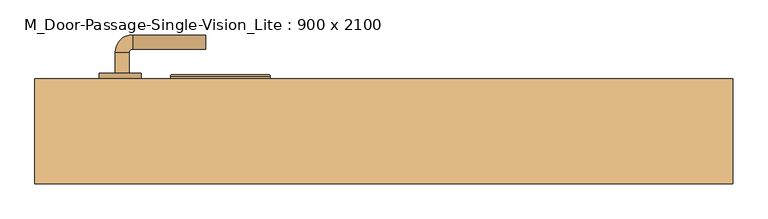
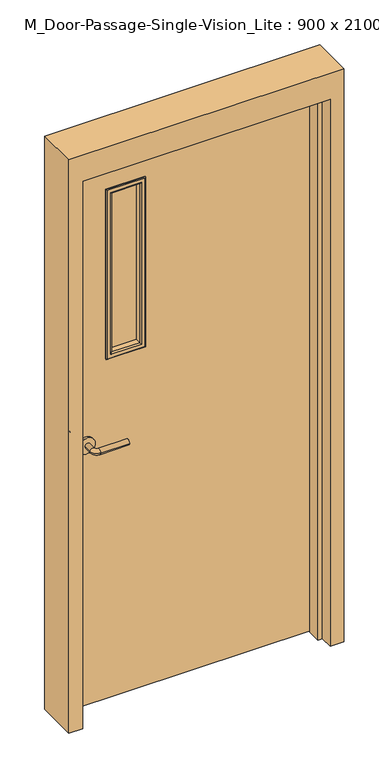
"""IFC4 building model written with IfcOpenShell, lengths in millimetres: door geometry, M_Door-Passage-Single-Vision_Lite : 900 x 2100."""

from ifc_helpers import new_model, si_unit, point, frame, frame_2d, origin, place, context, project, spatial, polyline, circle_curve, ellipse_curve, trimmed, segment, composite_curve, outline, extrude, faceted_brep, source, transform, mapped, element, save
from ifc_brep_helpers import plane_surface, cylinder_surface, revolved_surface, advanced_brep


def m_door_passage_single_vision_lite_900_x_2100_15962226(model_context):
    return source(origin(), model_context, "Body", "SolidModel", [
        advanced_brep(
        [(-384.990625, 40.85, 1000.0), (-364.990625, 40.85, 1000.0), (-364.990625, 10.85, 1000.0), (-384.990625, 10.85, 1000.0), (-359.990625, 5.85, 1000.0), (-359.990625, -14.15, 1000.0), (-254.990625, -14.15, 1000.0), (-254.990625, 5.85, 1000.0)],
        [
            (0, 1, circle_curve(frame((-374.990625, 40.85, 1000.0), z_axis=(0.0, 1.0, 0.0), x_axis=(1.0, 0.0, 0.0)), 10.0)),
            (1, 0, circle_curve(frame((-374.990625, 40.85, 1000.0), z_axis=(0.0, 1.0, 0.0), x_axis=(1.0, 0.0, 0.0)), 10.0)),
            (1, 2),
            (2, 3, circle_curve(frame((-374.990625, 10.85, 1000.0), z_axis=(0.0, 1.0, 0.0), x_axis=(1.0, 0.0, 0.0)), 10.0)),
            (3, 0),
            (3, 2, circle_curve(frame((-374.990625, 10.85, 1000.0), z_axis=(0.0, 1.0, 0.0), x_axis=(1.0, 0.0, 0.0)), 10.0)),
            (4, 5, circle_curve(frame((-359.990625, -4.15, 1000.0), z_axis=(-1.0, 0.0, 0.0), x_axis=(0.0, 1.0, 0.0)), 10.0)),
            (5, 3, circle_curve(frame((-359.990625, 10.85, 1000.0), z_axis=(0.0, 0.0, -1.0), x_axis=(-1.0, 0.0, 0.0)), 25.0)),
            (2, 4, circle_curve(frame((-359.990625, 10.85, 1000.0), z_axis=(0.0, 0.0, 1.0), x_axis=(-1.0, 0.0, 0.0)), 5.0)),
            (5, 4, circle_curve(frame((-359.990625, -4.15, 1000.0), z_axis=(-1.0, 0.0, 0.0), x_axis=(0.0, 1.0, 0.0)), 10.0)),
            (6, 7, circle_curve(frame((-254.990625, -4.15, 1000.0), z_axis=(1.0, 0.0, 0.0), x_axis=(0.0, 1.0, 0.0)), 10.0)),
            (7, 6, circle_curve(frame((-254.990625, -4.15, 1000.0), z_axis=(1.0, 0.0, 0.0), x_axis=(0.0, 1.0, 0.0)), 10.0)),
            (4, 7),
            (6, 5),
        ],
        [
            plane_surface(frame((-374.990625, 40.85, 1000.0), z_axis=(0.0, 1.0, 0.0), x_axis=(0.0, 0.0, 1.0))),
            cylinder_surface(frame((-374.990625, 40.85, 1000.0), z_axis=(0.0, 1.0, 0.0), x_axis=(1.0, 0.0, 0.0)), 10.0),
            revolved_surface(trimmed(ellipse_curve(frame((-374.990625, 10.85, 1000.0), z_axis=(0.0, -1.0, 0.0), x_axis=(1.0, 0.0, 0.0)), 10.0, 10.0), [point((-384.990625, 10.85, 1000.0))], [point((-364.990625, 10.85, 1000.0))], True, "CARTESIAN"), (-359.990625, 10.85, 1000.0), (0.0, 0.0, -1.0)),
            revolved_surface(trimmed(ellipse_curve(frame((-374.990625, 10.85, 1000.0), z_axis=(0.0, -1.0, 0.0), x_axis=(1.0, 0.0, 0.0)), 10.0, 10.0), [point((-364.990625, 10.85, 1000.0))], [point((-384.990625, 10.85, 1000.0))], True, "CARTESIAN"), (-359.990625, 10.85, 1000.0), (0.0, 0.0, -1.0)),
            plane_surface(frame((-254.990625, -4.15, 1000.0), z_axis=(1.0, 0.0, 0.0), x_axis=(0.0, 0.0, 1.0))),
            cylinder_surface(frame((-359.990625, -4.15, 1000.0), z_axis=(-1.0, 0.0, 0.0), x_axis=(0.0, 1.0, 0.0)), 10.0),
        ],
        [
            (0, [[1, 2]]),
            (1, [[3, 4, 5, -2]]),
            (1, [[-5, 6, -3, -1]]),
            (2, [[7, 8, -4, 9]]),
            (3, [[10, -9, -6, -8]]),
            (4, [[11, 12]]),
            (5, [[13, -11, 14, -7]]),
            (5, [[-14, -12, -13, -10]]),
        ],
    ),
        extrude(outline(composite_curve([segment(trimmed(circle_curve(frame_2d((1000.0, -377.490625)), 30.0), [point((1000.0, -407.490625))], [point((1000.0, -347.490625))], False, "CARTESIAN"), True, "CONTINUOUS"), segment(trimmed(circle_curve(frame_2d((1000.0, -377.490625)), 30.0), [point((1000.0, -347.490625))], [point((1000.0, -407.490625))], False, "CARTESIAN"), True, "CONTINUOUS")], self_intersect=False)), frame((0.0, 40.85, 0.0), z_axis=(0.0, 1.0, 0.0), x_axis=(0.0, 0.0, 1.0)), (0.0, 0.0, 1.0), 8.0),
        advanced_brep(
        [(-384.990625, 101.85, 1000.0), (-364.990625, 101.85, 1000.0), (-384.990625, 131.85, 1000.0), (-364.990625, 131.85, 1000.0), (-359.990625, 136.85, 1000.0), (-359.990625, 156.85, 1000.0), (-254.990625, 156.85, 1000.0), (-254.990625, 136.85, 1000.0)],
        [
            (0, 1, circle_curve(frame((-374.990625, 101.85, 1000.0), z_axis=(0.0, -1.0, 0.0), x_axis=(1.0, 0.0, 0.0)), 10.0)),
            (1, 0, circle_curve(frame((-374.990625, 101.85, 1000.0), z_axis=(0.0, -1.0, 0.0), x_axis=(1.0, 0.0, 0.0)), 10.0)),
            (0, 2),
            (2, 3, circle_curve(frame((-374.990625, 131.85, 1000.0), z_axis=(0.0, -1.0, 0.0), x_axis=(1.0, 0.0, 0.0)), 10.0)),
            (3, 1),
            (3, 2, circle_curve(frame((-374.990625, 131.85, 1000.0), z_axis=(0.0, -1.0, 0.0), x_axis=(1.0, 0.0, 0.0)), 10.0)),
            (4, 3, circle_curve(frame((-359.990625, 131.85, 1000.0), z_axis=(0.0, 0.0, 1.0), x_axis=(-1.0, 0.0, 0.0)), 5.0)),
            (2, 5, circle_curve(frame((-359.990625, 131.85, 1000.0), z_axis=(0.0, 0.0, -1.0), x_axis=(-1.0, 0.0, 0.0)), 25.0)),
            (5, 4, circle_curve(frame((-359.990625, 146.85, 1000.0), z_axis=(-1.0, 0.0, 0.0), x_axis=(0.0, -1.0, 0.0)), 10.0)),
            (4, 5, circle_curve(frame((-359.990625, 146.85, 1000.0), z_axis=(-1.0, 0.0, 0.0), x_axis=(0.0, -1.0, 0.0)), 10.0)),
            (6, 7, circle_curve(frame((-254.990625, 146.85, 1000.0), z_axis=(1.0, 0.0, 0.0), x_axis=(0.0, -1.0, 0.0)), 10.0)),
            (7, 6, circle_curve(frame((-254.990625, 146.85, 1000.0), z_axis=(1.0, 0.0, 0.0), x_axis=(0.0, -1.0, 0.0)), 10.0)),
            (5, 6),
            (7, 4),
        ],
        [
            plane_surface(frame((-374.990625, 101.85, 1000.0), z_axis=(0.0, -1.0, 0.0), x_axis=(0.0, 0.0, 1.0))),
            cylinder_surface(frame((-374.990625, 101.85, 1000.0), z_axis=(0.0, -1.0, 0.0), x_axis=(1.0, 0.0, 0.0)), 10.0),
            revolved_surface(trimmed(ellipse_curve(frame((-374.990625, 131.85, 1000.0), z_axis=(0.0, -1.0, 0.0), x_axis=(1.0, 0.0, 0.0)), 10.0, 10.0), [point((-384.990625, 131.85, 1000.0))], [point((-364.990625, 131.85, 1000.0))], True, "CARTESIAN"), (-359.990625, 131.85, 1000.0), (0.0, 0.0, -1.0)),
            revolved_surface(trimmed(ellipse_curve(frame((-374.990625, 131.85, 1000.0), z_axis=(0.0, -1.0, 0.0), x_axis=(1.0, 0.0, 0.0)), 10.0, 10.0), [point((-364.990625, 131.85, 1000.0))], [point((-384.990625, 131.85, 1000.0))], True, "CARTESIAN"), (-359.990625, 131.85, 1000.0), (0.0, 0.0, -1.0)),
            plane_surface(frame((-254.990625, 146.85, 1000.0), z_axis=(1.0, 0.0, 0.0), x_axis=(0.0, 0.0, 1.0))),
            cylinder_surface(frame((-359.990625, 146.85, 1000.0), z_axis=(-1.0, 0.0, 0.0), x_axis=(0.0, -1.0, 0.0)), 10.0),
        ],
        [
            (0, [[1, 2]]),
            (1, [[-1, 3, 4, 5]]),
            (1, [[-2, -5, 6, -3]]),
            (2, [[7, -4, 8, 9]]),
            (3, [[-8, -6, -7, 10]]),
            (4, [[11, 12]]),
            (5, [[-9, 13, -12, 14]]),
            (5, [[-10, -14, -11, -13]]),
        ],
    ),
        extrude(outline(composite_curve([segment(trimmed(circle_curve(frame_2d((1000.0, -377.490625)), 30.0), [point((1000.0, -407.490625))], [point((1000.0, -347.490625))], False, "CARTESIAN"), True, "CONTINUOUS"), segment(trimmed(circle_curve(frame_2d((1000.0, -377.490625)), 30.0), [point((1000.0, -347.490625))], [point((1000.0, -407.490625))], False, "CARTESIAN"), True, "CONTINUOUS")], self_intersect=False)), frame((0.0, 93.85, 0.0), z_axis=(0.0, 1.0, 0.0), x_axis=(0.0, 0.0, 1.0)), (0.0, 0.0, 1.0), 8.0),
        extrude(outline(polyline([(2100.0, -450.0), (0.0, -450.0), (0.0, 450.0), (2100.0, 450.0), (2100.0, -450.0)]), holes=[polyline([(1947.6, -297.6), (1947.6, -170.6), (1312.6, -170.6), (1312.6, -297.6), (1947.6, -297.6)])]), frame((0.0, 48.85, 0.0), z_axis=(0.0, 1.0, 0.0), x_axis=(0.0, 0.0, 1.0)), (0.0, 0.0, 1.0), 45.0),
        faceted_brep([(450.0, 44.0875, 0.0), (450.0, 93.85, 0.0), (500.0, 93.85, 0.0), (500.0, -56.15, 0.0), (450.0, -56.15, 0.0), (450.0, -6.9375, 0.0), (434.125, -6.9375, 0.0), (434.125, 44.0875, 0.0), (450.0, 44.0875, 2100.0), (450.0, 93.85, 2100.0), (-450.0, 93.85, 2100.0), (-450.0, 93.85, 0.0), (-500.0, 93.85, 0.0), (-500.0, 93.85, 2200.0), (500.0, 93.85, 2200.0), (500.0, -56.15, 2200.0), (-500.0, -56.15, 2200.0), (-500.0, -56.15, 0.0), (-450.0, -56.15, 0.0), (-450.0, -56.15, 2100.0), (450.0, -56.15, 2100.0), (450.0, -6.9375, 2100.0), (-450.0, -6.9375, 2100.0), (-450.0, -6.9375, 0.0), (-434.125, -6.9375, 0.0), (-434.125, -6.9375, 2084.125), (434.125, -6.9375, 2084.125), (434.125, 44.0875, 2084.125), (-434.125, 44.0875, 2084.125), (-434.125, 44.0875, 0.0), (-450.0, 44.0875, 0.0), (-450.0, 44.0875, 2100.0)], [[[0, 1, 2, 3, 4, 5, 6, 7]], [[1, 0, 8, 9]], [[2, 1, 9, 10, 11, 12, 13, 14]], [[3, 2, 14, 15]], [[4, 3, 15, 16, 17, 18, 19, 20]], [[5, 4, 20, 21]], [[6, 5, 21, 22, 23, 24, 25, 26]], [[7, 6, 26, 27]], [[0, 7, 27, 28, 29, 30, 31, 8]], [[9, 8, 31, 10]], [[20, 19, 22, 21]], [[26, 25, 28, 27]], [[12, 11, 30, 29, 24, 23, 18, 17]], [[11, 10, 31, 30]], [[13, 12, 17, 16]], [[19, 18, 23, 22]], [[25, 24, 29, 28]], [[15, 14, 13, 16]]]),
        extrude(outline(polyline([(-170.6, 68.85), (-297.6, 68.85), (-297.6, 73.85), (-170.6, 73.85), (-170.6, 68.85)])), frame((0.0, 0.0, 1312.6), z_axis=(0.0, 0.0, 1.0), x_axis=(1.0, 0.0, 0.0)), (0.0, 0.0, 1.0), 635.0),
        advanced_brep(
        [(-297.6, 73.85, 1947.6), (-297.6, 93.85, 1947.6), (-297.6, 93.85, 1312.6), (-297.6, 73.85, 1312.6), (-285.6, 94.85, 1935.6), (-285.6, 73.85, 1935.6), (-285.6, 73.85, 1324.6), (-285.6, 94.85, 1324.6), (-290.6, 99.85, 1940.6), (-290.6, 99.85, 1319.6), (-305.6, 97.85, 1955.6), (-303.6, 99.85, 1953.6), (-303.6, 99.85, 1306.6), (-305.6, 97.85, 1304.6), (-305.6, 93.85, 1955.6), (-305.6, 93.85, 1304.6), (-170.6, 93.85, 1312.6), (-170.6, 73.85, 1312.6), (-182.6, 73.85, 1324.6), (-182.6, 94.85, 1324.6), (-177.6, 99.85, 1319.6), (-164.6, 99.85, 1306.6), (-162.6, 97.85, 1304.6), (-162.6, 93.85, 1304.6), (-170.6, 93.85, 1947.6), (-170.6, 73.85, 1947.6), (-182.6, 73.85, 1935.6), (-182.6, 94.85, 1935.6), (-177.6, 99.85, 1940.6), (-164.6, 99.85, 1953.6), (-162.6, 97.85, 1955.6), (-162.6, 93.85, 1955.6)],
        [
            (0, 1),
            (1, 2),
            (2, 3),
            (3, 0),
            (4, 5),
            (5, 6),
            (6, 7),
            (7, 4),
            (8, 4, ellipse_curve(frame((-290.6, 94.85, 1940.6), z_axis=(-0.7071067811865475, 0.0, -0.7071067811865475), x_axis=(-0.7071067811865474, 0.0, 0.7071067811865476)), 7.0710678, 5.0)),
            (7, 9, ellipse_curve(frame((-290.6, 94.85, 1319.6), z_axis=(-0.7071067811865475, 0.0, 0.7071067811865475), x_axis=(0.7071067811865474, 0.0, 0.7071067811865476)), 7.0710678, 5.0)),
            (9, 8),
            (10, 11, ellipse_curve(frame((-303.6, 97.85, 1953.6), z_axis=(-0.7071067811865475, 0.0, -0.7071067811865475), x_axis=(-0.7071067811865474, 0.0, 0.7071067811865476)), 2.8284271, 2.0)),
            (11, 12),
            (12, 13, ellipse_curve(frame((-303.6, 97.85, 1306.6), z_axis=(-0.7071067811865475, 0.0, 0.7071067811865475), x_axis=(0.7071067811865474, 0.0, 0.7071067811865476)), 2.8284271, 2.0)),
            (13, 10),
            (14, 10),
            (13, 15),
            (15, 14),
            (2, 16),
            (16, 17),
            (17, 3),
            (6, 18),
            (18, 19),
            (19, 7),
            (19, 20, ellipse_curve(frame((-177.6, 94.85, 1319.6), z_axis=(-0.7071067811865475, 0.0, -0.7071067811865475), x_axis=(-0.7071067811865476, 0.0, 0.7071067811865474)), 7.0710678, 5.0)),
            (20, 9),
            (12, 21),
            (21, 22, ellipse_curve(frame((-164.6, 97.85, 1306.6), z_axis=(-0.7071067811865475, 0.0, -0.7071067811865475), x_axis=(-0.7071067811865476, 0.0, 0.7071067811865474)), 2.8284271, 2.0)),
            (22, 13),
            (22, 23),
            (23, 15),
            (16, 24),
            (24, 25),
            (25, 17),
            (18, 26),
            (26, 27),
            (27, 19),
            (27, 28, ellipse_curve(frame((-177.6, 94.85, 1940.6), z_axis=(0.7071067811865475, 0.0, -0.7071067811865475), x_axis=(-0.7071067811865474, 0.0, -0.7071067811865476)), 7.0710678, 5.0)),
            (28, 20),
            (21, 29),
            (29, 30, ellipse_curve(frame((-164.6, 97.85, 1953.6), z_axis=(0.7071067811865475, 0.0, -0.7071067811865475), x_axis=(-0.7071067811865474, 0.0, -0.7071067811865476)), 2.8284271, 2.0)),
            (30, 22),
            (30, 31),
            (31, 23),
            (31, 14),
            (1, 24),
            (0, 25),
            (5, 26),
            (4, 27),
            (8, 28),
            (11, 29),
            (10, 30),
        ],
        [
            plane_surface(frame((-297.6, 93.85, 1947.6), z_axis=(-1.0, 0.0, 0.0), x_axis=(0.0, 0.0, -1.0))),
            plane_surface(frame((-285.6, 73.85, 1935.6), z_axis=(1.0, 0.0, 0.0), x_axis=(0.0, 0.0, -1.0))),
            cylinder_surface(frame((-290.6, 94.85, 1947.6), z_axis=(0.0, 0.0, 1.0), x_axis=(-1.0, 0.0, 0.0)), 5.0),
            cylinder_surface(frame((-303.6, 97.85, 1947.6), z_axis=(0.0, 0.0, 1.0), x_axis=(-1.0, 0.0, 0.0)), 2.0),
            plane_surface(frame((-305.6, 97.85, 1955.6), z_axis=(-1.0, 0.0, 0.0), x_axis=(0.0, 0.0, -1.0))),
            plane_surface(frame((-297.6, 93.85, 1312.6), z_axis=(0.0, 0.0, -1.0), x_axis=(1.0, 0.0, 0.0))),
            plane_surface(frame((-285.6, 73.85, 1324.6), z_axis=(0.0, 0.0, 1.0), x_axis=(1.0, 0.0, 0.0))),
            cylinder_surface(frame((-297.6, 94.85, 1319.6), z_axis=(-1.0, 0.0, 0.0), x_axis=(0.0, 0.0, -1.0)), 5.0),
            cylinder_surface(frame((-297.6, 97.85, 1306.6), z_axis=(-1.0, 0.0, 0.0), x_axis=(0.0, 0.0, -1.0)), 2.0),
            plane_surface(frame((-305.6, 97.85, 1304.6), z_axis=(0.0, 0.0, -1.0), x_axis=(1.0, 0.0, 0.0))),
            plane_surface(frame((-170.6, 93.85, 1312.6), z_axis=(1.0, 0.0, 0.0), x_axis=(0.0, 0.0, 1.0))),
            plane_surface(frame((-182.6, 73.85, 1324.6), z_axis=(-1.0, 0.0, 0.0), x_axis=(0.0, 0.0, 1.0))),
            cylinder_surface(frame((-177.6, 94.85, 1312.6), z_axis=(0.0, 0.0, -1.0), x_axis=(1.0, 0.0, 0.0)), 5.0),
            cylinder_surface(frame((-164.6, 97.85, 1312.6), z_axis=(0.0, 0.0, -1.0), x_axis=(1.0, 0.0, 0.0)), 2.0),
            plane_surface(frame((-162.6, 97.85, 1304.6), z_axis=(1.0, 0.0, 0.0), x_axis=(0.0, 0.0, 1.0))),
            plane_surface(frame((-162.6, 93.85, 1955.6), z_axis=(0.0, -1.0, 0.0), x_axis=(-1.0, 0.0, 0.0))),
            plane_surface(frame((-170.6, 93.85, 1947.6), z_axis=(0.0, 0.0, 1.0), x_axis=(-1.0, 0.0, 0.0))),
            plane_surface(frame((-170.6, 73.85, 1947.6), z_axis=(0.0, -1.0, 0.0), x_axis=(-1.0, 0.0, 0.0))),
            plane_surface(frame((-182.6, 73.85, 1935.6), z_axis=(0.0, 0.0, -1.0), x_axis=(-1.0, 0.0, 0.0))),
            cylinder_surface(frame((-170.6, 94.85, 1940.6), z_axis=(1.0, 0.0, 0.0), x_axis=(0.0, 0.0, 1.0)), 5.0),
            plane_surface(frame((-177.6, 99.85, 1940.6), z_axis=(0.0, 1.0, 0.0), x_axis=(-1.0, 0.0, 0.0))),
            cylinder_surface(frame((-170.6, 97.85, 1953.6), z_axis=(1.0, 0.0, 0.0), x_axis=(0.0, 0.0, 1.0)), 2.0),
            plane_surface(frame((-162.6, 97.85, 1955.6), z_axis=(0.0, 0.0, 1.0), x_axis=(-1.0, 0.0, 0.0))),
        ],
        [
            (0, [[1, 2, 3, 4]]),
            (1, [[5, 6, 7, 8]]),
            (2, [[9, -8, 10, 11]]),
            (3, [[12, 13, 14, 15]]),
            (4, [[16, -15, 17, 18]]),
            (5, [[-3, 19, 20, 21]]),
            (6, [[-7, 22, 23, 24]]),
            (7, [[-10, -24, 25, 26]]),
            (8, [[-14, 27, 28, 29]]),
            (9, [[-17, -29, 30, 31]]),
            (10, [[-20, 32, 33, 34]]),
            (11, [[-23, 35, 36, 37]]),
            (12, [[-25, -37, 38, 39]]),
            (13, [[-28, 40, 41, 42]]),
            (14, [[-30, -42, 43, 44]]),
            (15, [[-31, -44, 45, -18], [46, -32, -19, -2]]),
            (16, [[-33, -46, -1, 47]]),
            (17, [[-21, -34, -47, -4], [48, -35, -22, -6]]),
            (18, [[-36, -48, -5, 49]]),
            (19, [[-38, -49, -9, 50]]),
            (20, [[51, -40, -27, -13], [-26, -39, -50, -11]]),
            (21, [[-41, -51, -12, 52]]),
            (22, [[-43, -52, -16, -45]]),
        ],
    ),
        advanced_brep(
        [(-297.6, 68.85, 1312.6), (-297.6, 48.85, 1312.6), (-297.6, 48.85, 1947.6), (-297.6, 68.85, 1947.6), (-285.6, 47.85, 1324.6), (-285.6, 68.85, 1324.6), (-285.6, 68.85, 1935.6), (-285.6, 47.85, 1935.6), (-290.6, 42.85, 1319.6), (-290.6, 42.85, 1940.6), (-305.6, 44.85, 1304.6), (-303.6, 42.85, 1306.6), (-303.6, 42.85, 1953.6), (-305.6, 44.85, 1955.6), (-305.6, 48.85, 1304.6), (-305.6, 48.85, 1955.6), (-170.6, 48.85, 1947.6), (-170.6, 68.85, 1947.6), (-182.6, 68.85, 1935.6), (-182.6, 47.85, 1935.6), (-177.6, 42.85, 1940.6), (-164.6, 42.85, 1953.6), (-162.6, 44.85, 1955.6), (-162.6, 48.85, 1955.6), (-170.6, 48.85, 1312.6), (-170.6, 68.85, 1312.6), (-182.6, 68.85, 1324.6), (-182.6, 47.85, 1324.6), (-177.6, 42.85, 1319.6), (-164.6, 42.85, 1306.6), (-162.6, 44.85, 1304.6), (-162.6, 48.85, 1304.6)],
        [
            (0, 1),
            (1, 2),
            (2, 3),
            (3, 0),
            (4, 5),
            (5, 6),
            (6, 7),
            (7, 4),
            (8, 4, ellipse_curve(frame((-290.6, 47.85, 1319.6), z_axis=(-0.7071067811865475, 0.0, 0.7071067811865475), x_axis=(-0.7071067811865474, 0.0, -0.7071067811865476)), 7.0710678, 5.0)),
            (7, 9, ellipse_curve(frame((-290.6, 47.85, 1940.6), z_axis=(-0.7071067811865475, 0.0, -0.7071067811865475), x_axis=(0.7071067811865474, 0.0, -0.7071067811865476)), 7.0710678, 5.0)),
            (9, 8),
            (10, 11, ellipse_curve(frame((-303.6, 44.85, 1306.6), z_axis=(-0.7071067811865475, 0.0, 0.7071067811865475), x_axis=(-0.7071067811865474, 0.0, -0.7071067811865476)), 2.8284271, 2.0)),
            (11, 12),
            (12, 13, ellipse_curve(frame((-303.6, 44.85, 1953.6), z_axis=(-0.7071067811865475, 0.0, -0.7071067811865475), x_axis=(0.7071067811865474, 0.0, -0.7071067811865476)), 2.8284271, 2.0)),
            (13, 10),
            (14, 10),
            (13, 15),
            (15, 14),
            (2, 16),
            (16, 17),
            (17, 3),
            (6, 18),
            (18, 19),
            (19, 7),
            (19, 20, ellipse_curve(frame((-177.6, 47.85, 1940.6), z_axis=(-0.7071067811865475, 0.0, 0.7071067811865475), x_axis=(-0.7071067811865476, 0.0, -0.7071067811865474)), 7.0710678, 5.0)),
            (20, 9),
            (12, 21),
            (21, 22, ellipse_curve(frame((-164.6, 44.85, 1953.6), z_axis=(-0.7071067811865475, 0.0, 0.7071067811865475), x_axis=(-0.7071067811865476, 0.0, -0.7071067811865474)), 2.8284271, 2.0)),
            (22, 13),
            (22, 23),
            (23, 15),
            (16, 24),
            (24, 25),
            (25, 17),
            (18, 26),
            (26, 27),
            (27, 19),
            (27, 28, ellipse_curve(frame((-177.6, 47.85, 1319.6), z_axis=(0.7071067811865475, 0.0, 0.7071067811865475), x_axis=(-0.7071067811865474, 0.0, 0.7071067811865476)), 7.0710678, 5.0)),
            (28, 20),
            (21, 29),
            (29, 30, ellipse_curve(frame((-164.6, 44.85, 1306.6), z_axis=(0.7071067811865475, 0.0, 0.7071067811865475), x_axis=(-0.7071067811865474, 0.0, 0.7071067811865476)), 2.8284271, 2.0)),
            (30, 22),
            (30, 31),
            (31, 23),
            (31, 14),
            (1, 24),
            (0, 25),
            (5, 26),
            (4, 27),
            (8, 28),
            (11, 29),
            (10, 30),
        ],
        [
            plane_surface(frame((-297.6, 48.85, 1312.6), z_axis=(-1.0, 0.0, 0.0), x_axis=(0.0, 0.0, 1.0))),
            plane_surface(frame((-285.6, 68.85, 1324.6), z_axis=(1.0, 0.0, 0.0), x_axis=(0.0, 0.0, 1.0))),
            cylinder_surface(frame((-290.6, 47.85, 1312.6), z_axis=(0.0, 0.0, -1.0), x_axis=(-1.0, 0.0, 0.0)), 5.0),
            cylinder_surface(frame((-303.6, 44.85, 1312.6), z_axis=(0.0, 0.0, -1.0), x_axis=(-1.0, 0.0, 0.0)), 2.0),
            plane_surface(frame((-305.6, 44.85, 1304.6), z_axis=(-1.0, 0.0, 0.0), x_axis=(0.0, 0.0, 1.0))),
            plane_surface(frame((-297.6, 48.85, 1947.6), z_axis=(0.0, 0.0, 1.0), x_axis=(1.0, 0.0, 0.0))),
            plane_surface(frame((-285.6, 68.85, 1935.6), z_axis=(0.0, 0.0, -1.0), x_axis=(1.0, 0.0, 0.0))),
            cylinder_surface(frame((-297.6, 47.85, 1940.6), z_axis=(-1.0, 0.0, 0.0), x_axis=(0.0, 0.0, 1.0)), 5.0),
            cylinder_surface(frame((-297.6, 44.85, 1953.6), z_axis=(-1.0, 0.0, 0.0), x_axis=(0.0, 0.0, 1.0)), 2.0),
            plane_surface(frame((-305.6, 44.85, 1955.6), z_axis=(0.0, 0.0, 1.0), x_axis=(1.0, 0.0, 0.0))),
            plane_surface(frame((-170.6, 48.85, 1947.6), z_axis=(1.0, 0.0, 0.0), x_axis=(0.0, 0.0, -1.0))),
            plane_surface(frame((-182.6, 68.85, 1935.6), z_axis=(-1.0, 0.0, 0.0), x_axis=(0.0, 0.0, -1.0))),
            cylinder_surface(frame((-177.6, 47.85, 1947.6), z_axis=(0.0, 0.0, 1.0), x_axis=(1.0, 0.0, 0.0)), 5.0),
            cylinder_surface(frame((-164.6, 44.85, 1947.6), z_axis=(0.0, 0.0, 1.0), x_axis=(1.0, 0.0, 0.0)), 2.0),
            plane_surface(frame((-162.6, 44.85, 1955.6), z_axis=(1.0, 0.0, 0.0), x_axis=(0.0, 0.0, -1.0))),
            plane_surface(frame((-162.6, 48.85, 1304.6), z_axis=(0.0, 1.0, 0.0), x_axis=(-1.0, 0.0, 0.0))),
            plane_surface(frame((-170.6, 48.85, 1312.6), z_axis=(0.0, 0.0, -1.0), x_axis=(-1.0, 0.0, 0.0))),
            plane_surface(frame((-170.6, 68.85, 1312.6), z_axis=(0.0, 1.0, 0.0), x_axis=(-1.0, 0.0, 0.0))),
            plane_surface(frame((-182.6, 68.85, 1324.6), z_axis=(0.0, 0.0, 1.0), x_axis=(-1.0, 0.0, 0.0))),
            cylinder_surface(frame((-170.6, 47.85, 1319.6), z_axis=(1.0, 0.0, 0.0), x_axis=(0.0, 0.0, -1.0)), 5.0),
            plane_surface(frame((-177.6, 42.85, 1319.6), z_axis=(0.0, -1.0, 0.0), x_axis=(-1.0, 0.0, 0.0))),
            cylinder_surface(frame((-170.6, 44.85, 1306.6), z_axis=(1.0, 0.0, 0.0), x_axis=(0.0, 0.0, -1.0)), 2.0),
            plane_surface(frame((-162.6, 44.85, 1304.6), z_axis=(0.0, 0.0, -1.0), x_axis=(-1.0, 0.0, 0.0))),
        ],
        [
            (0, [[1, 2, 3, 4]]),
            (1, [[5, 6, 7, 8]]),
            (2, [[9, -8, 10, 11]]),
            (3, [[12, 13, 14, 15]]),
            (4, [[16, -15, 17, 18]]),
            (5, [[-3, 19, 20, 21]]),
            (6, [[-7, 22, 23, 24]]),
            (7, [[-10, -24, 25, 26]]),
            (8, [[-14, 27, 28, 29]]),
            (9, [[-17, -29, 30, 31]]),
            (10, [[-20, 32, 33, 34]]),
            (11, [[-23, 35, 36, 37]]),
            (12, [[-25, -37, 38, 39]]),
            (13, [[-28, 40, 41, 42]]),
            (14, [[-30, -42, 43, 44]]),
            (15, [[-31, -44, 45, -18], [46, -32, -19, -2]]),
            (16, [[-33, -46, -1, 47]]),
            (17, [[-21, -34, -47, -4], [48, -35, -22, -6]]),
            (18, [[-36, -48, -5, 49]]),
            (19, [[-38, -49, -9, 50]]),
            (20, [[51, -40, -27, -13], [-26, -39, -50, -11]]),
            (21, [[-41, -51, -12, 52]]),
            (22, [[-43, -52, -16, -45]]),
        ],
    ),
    ])


if __name__ == "__main__":
    model = new_model("IFC4")
    model_context = context("Model", 3, world=origin())
    ifc_project = project(units=[si_unit("LENGTHUNIT", "METRE", prefix="MILLI")], contexts=[model_context])
    site = spatial("IfcSite", under=ifc_project)
    building = spatial("IfcBuilding", under=site)
    placement = place(None, origin())
    m_door_passage_single_vision_lite_900_x_2100_shape = m_door_passage_single_vision_lite_900_x_2100_15962226(model_context)
    element("IfcDoor", 1, ObjectType="M_Door-Passage-Single-Vision_Lite : 900 x 2100", at=placement, inside=building, context=model_context, shape_type="MappedRepresentation", body=[
        mapped(m_door_passage_single_vision_lite_900_x_2100_shape, transform((0.0, 0.0, 0.0), x_axis=(1.0, 0.0, 0.0), y_axis=(0.0, 1.0, 0.0), z_axis=(0.0, 0.0, 1.0))),
    ])
    save(model, "model.ifc")

# Revit data of these elements
# Type "M_Door-Passage-Single-Vision_Lite : 900 x 2100"
#   Type Mark = "46"
#   Assembly Code = "B2030100"
#   Analytic Construction = "Wooden"
#   Thickness = 45 mm
#   Thermal Resistance (R) = 0.455703 (m²·K)/W
#   Swing Angle [instance default] = 90.00°
#   Strike Height = 1000 mm
#   Rough Width [instance default] = 1000 mm
#   Rough Height [instance default] = 2200 mm
#   MFOpeningHeight [instance default] = 100 mm
#   MFOpeningWidth [instance default] = 100 mm
#   Inset Calculate [instance default] = 105 mm
#   Masonry Inset [instance default] = 25 mm
#   Height = 2100 mm
#   Width = 900 mm
#   Heat Transfer Coefficient (U) = 2.19465 W/(m²·K)
#   Masonry Frame Depth = 150 mm
#   Masonry Frame [instance default] = yes
#   Function = 1
#   Dry Wall Frame [instance default] = no
#   Panel Material = Wood - Birch
#   Glazing = Glass
#   Glass Stop Material = Metal - Paint Finish - Grey
#   Frame Material = Metal - Paint Finish - Grey
#   Door Handle Material = Aluminum
#   Visual Light Transmittance = 0
#   Solar Heat Gain Coefficient = 0
#   Wall Closure = (empty or 0)
# Element 1 (IfcDoor, "M_Door-Passage-Single-Vision_Lite : 900 x 2100")
#   Materials on its faces: "Metal - Paint Finish - Grey", "Aluminum", "Wood - Birch", "Glass"
# Materials
#   "Wood - Birch": class "Wood", colour RGB 173 132 96, transparency 0, Cost = 0
#   "Glass": class "Glass", colour RGB 245 245 243, transparency 1, Description = "Soda Lime Glass", Cost = 0
#   "Metal - Paint Finish - Grey": class "Paint", colour RGB 178 178 178, transparency 0, Cost = 0
#   "Aluminum": class "Metal", colour RGB 244 245 246, transparency 0, Description = "Aluminum 6061", Cost = 0
